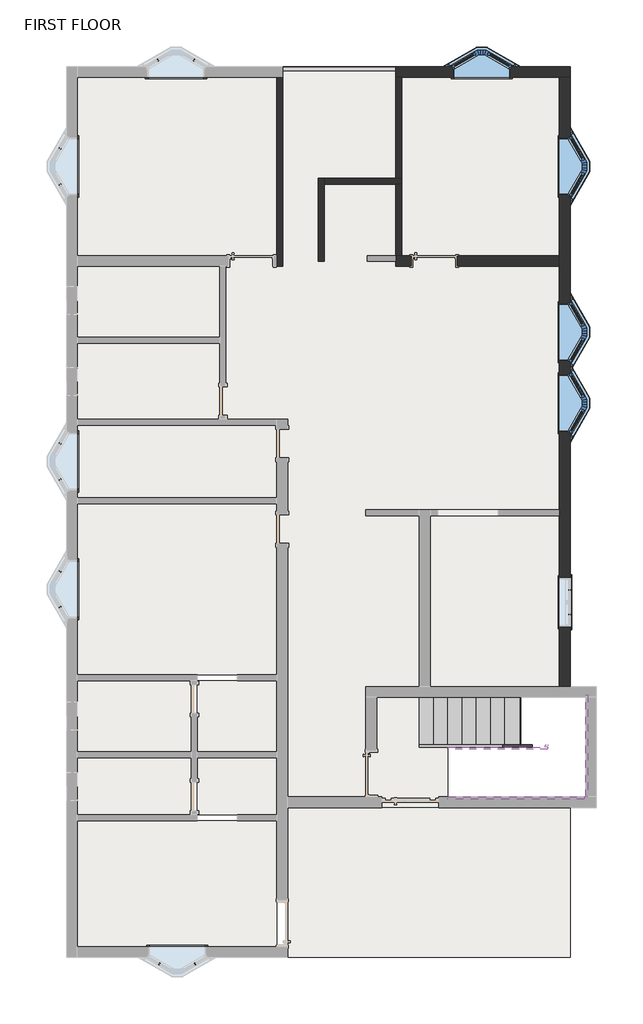
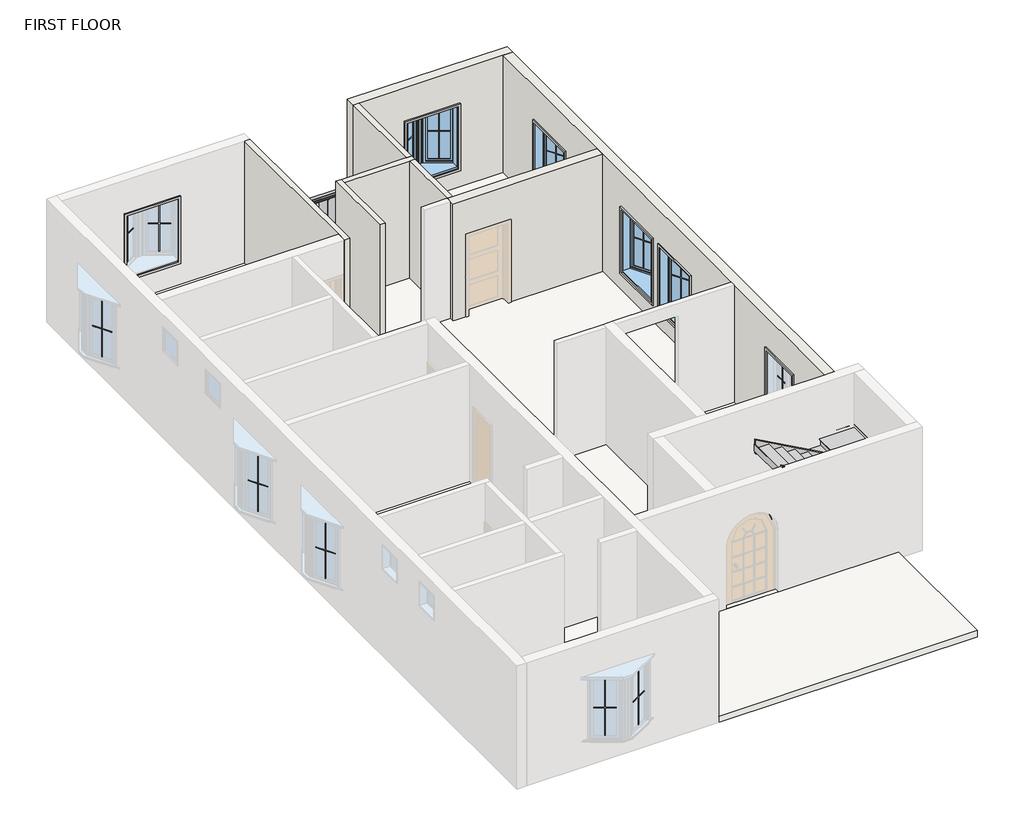
# One storey, part 2 of 2: 31 proxies, 8 walls, 6 members, 4 windows, 3 slabs, 1 railing, 1 stair flight.
"""IFC4 building model written with IfcOpenShell, lengths in millimetres."""

from ifc_helpers import new_model, si_unit, point, frame, origin, place, context, project, spatial, polyline, ellipse_curve, trimmed, outline, extrude, faceted_brep, transform, mapped, element, save
from ifc_brep_helpers import plane_surface, extruded_surface, advanced_brep
from components import muntin_pattern_2x2_muntin_pattern_2x2_75bf01dd, muntin_pattern_2x2_muntin_pattern_2x2_32baafd4, muntin_pattern_2x2_muntin_pattern_2x2_88bf7f41, muntin_pattern_2x2_muntin_pattern_2x2_3dfd0a47, trim_window_exterior_flat_with_sill_4930676f, trim_window_interior_flat_picture_frame_1060724f, trim_window_interior_flat_picture_frame_dd064338, stair_flight_7f10be43, window_bay_casement_30_degree_angle_30_angle_window_doors_2_b97d1700

model = new_model("IFC4")

# Units and contexts
model_context = context("Model", 3, world=origin())
ifc_project = project(units=[si_unit("LENGTHUNIT", "METRE", prefix="MILLI")], contexts=[model_context])

# Site, building, storey
site = spatial("IfcSite", under=ifc_project)
building = spatial("IfcBuilding", under=site)
storey = spatial("IfcBuildingStorey", under=building, Name="FIRST FLOOR", Elevation=3352.8)

# Proxies
placement = place(None, origin())
muntin_pattern_2x2_muntin_pattern_2x2_shape = muntin_pattern_2x2_muntin_pattern_2x2_75bf01dd(model_context)
element("IfcBuildingElementProxy", 1, Name="Muntin Pattern_2x2 : Muntin Pattern_2x2", ObjectType="Muntin Pattern_2x2 : Muntin Pattern_2x2", at=placement, inside=storey, context=model_context, shape_type="MappedRepresentation", body=[
    mapped(muntin_pattern_2x2_muntin_pattern_2x2_shape, transform((-20440.5197687, 51.8003691, 4083.05), x_axis=(-0.49999999999999245, 0.866025403784443, 0.0), y_axis=(-0.866025403784443, -0.49999999999999245, 0.0), z_axis=(0.0, 0.0, 1.0))),
])
element("IfcBuildingElementProxy", 2, Name="Muntin Pattern_2x2 : Muntin Pattern_2x2", ObjectType="Muntin Pattern_2x2 : Muntin Pattern_2x2", at=placement, inside=storey, context=model_context, shape_type="MappedRepresentation", body=[
    mapped(muntin_pattern_2x2_muntin_pattern_2x2_shape, transform((-20440.5197687, 2782.3003691, 4083.05), x_axis=(-0.49999999999999245, 0.866025403784443, 0.0), y_axis=(-0.866025403784443, -0.49999999999999245, 0.0), z_axis=(0.0, 0.0, 1.0))),
])
element("IfcBuildingElementProxy", 3, Name="Muntin Pattern_2x2 : Muntin Pattern_2x2", ObjectType="Muntin Pattern_2x2 : Muntin Pattern_2x2", at=placement, inside=storey, context=model_context, shape_type="MappedRepresentation", body=[
    mapped(muntin_pattern_2x2_muntin_pattern_2x2_shape, transform((-20440.5197687, 9094.2003691, 4083.05), x_axis=(-0.49999999999999245, 0.866025403784443, 0.0), y_axis=(-0.866025403784443, -0.49999999999999245, 0.0), z_axis=(0.0, 0.0, 1.0))),
])
element("IfcBuildingElementProxy", 4, Name="Muntin Pattern_2x2 : Muntin Pattern_2x2", ObjectType="Muntin Pattern_2x2 : Muntin Pattern_2x2", at=placement, inside=storey, context=model_context, shape_type="MappedRepresentation", body=[
    mapped(muntin_pattern_2x2_muntin_pattern_2x2_shape, transform((-18344.0408789, 11750.0736953, 4083.05), x_axis=(0.866025403784444, 0.49999999999999084, 0.0), y_axis=(-0.49999999999999084, 0.866025403784444, 0.0), z_axis=(0.0, 0.0, 1.0))),
])
element("IfcBuildingElementProxy", 5, Name="Muntin Pattern_2x2 : Muntin Pattern_2x2", ObjectType="Muntin Pattern_2x2 : Muntin Pattern_2x2", at=placement, inside=storey, context=model_context, shape_type="MappedRepresentation", body=[
    mapped(muntin_pattern_2x2_muntin_pattern_2x2_shape, transform((-11803.5408789, 11750.0736953, 4083.05), x_axis=(0.866025403784444, 0.49999999999999084, 0.0), y_axis=(-0.49999999999999084, 0.866025403784444, 0.0), z_axis=(0.0, 0.0, 1.0))),
])
element("IfcBuildingElementProxy", 6, Name="Muntin Pattern_2x2 : Muntin Pattern_2x2", ObjectType="Muntin Pattern_2x2 : Muntin Pattern_2x2", at=placement, inside=storey, context=model_context, shape_type="MappedRepresentation", body=[
    mapped(muntin_pattern_2x2_muntin_pattern_2x2_shape, transform((-9388.9675526, 9856.7948055, 4083.05), x_axis=(0.49999999999999245, -0.866025403784443, 0.0), y_axis=(0.866025403784443, 0.49999999999999245, 0.0), z_axis=(0.0, 0.0, 1.0))),
])
element("IfcBuildingElementProxy", 7, Name="Muntin Pattern_2x2 : Muntin Pattern_2x2", ObjectType="Muntin Pattern_2x2 : Muntin Pattern_2x2", at=placement, inside=storey, context=model_context, shape_type="MappedRepresentation", body=[
    mapped(muntin_pattern_2x2_muntin_pattern_2x2_shape, transform((-9388.9675526, 6313.4948055, 4083.05), x_axis=(0.49999999999999245, -0.866025403784443, 0.0), y_axis=(0.866025403784443, 0.49999999999999245, 0.0), z_axis=(0.0, 0.0, 1.0))),
])
element("IfcBuildingElementProxy", 8, Name="Muntin Pattern_2x2 : Muntin Pattern_2x2", ObjectType="Muntin Pattern_2x2 : Muntin Pattern_2x2", at=placement, inside=storey, context=model_context, shape_type="MappedRepresentation", body=[
    mapped(muntin_pattern_2x2_muntin_pattern_2x2_shape, transform((-9388.9675526, 4789.4948055, 4083.05), x_axis=(0.49999999999999245, -0.866025403784443, 0.0), y_axis=(0.866025403784443, 0.49999999999999245, 0.0), z_axis=(0.0, 0.0, 1.0))),
])
element("IfcBuildingElementProxy", 9, Name="Muntin Pattern_2x2 : Muntin Pattern_2x2", ObjectType="Muntin Pattern_2x2 : Muntin Pattern_2x2", at=placement, inside=storey, context=model_context, shape_type="MappedRepresentation", body=[
    mapped(muntin_pattern_2x2_muntin_pattern_2x2_shape, transform((-17556.0464424, -7581.8785207, 4083.05), x_axis=(-0.8660254037844438, -0.49999999999999106, 0.0), y_axis=(0.49999999999999106, -0.8660254037844438, 0.0), z_axis=(0.0, 0.0, 1.0))),
])
muntin_pattern_2x2_muntin_pattern_2x2_2_shape = muntin_pattern_2x2_muntin_pattern_2x2_32baafd4(model_context)
element("IfcBuildingElementProxy", 10, Name="Muntin Pattern_2x2 : Muntin Pattern_2x2", ObjectType="Muntin Pattern_2x2 : Muntin Pattern_2x2", at=placement, inside=storey, context=model_context, shape_type="MappedRepresentation", body=[
    mapped(muntin_pattern_2x2_muntin_pattern_2x2_2_shape, transform((-20440.5197687, 814.3948055, 4083.05), x_axis=(-0.4999999999999952, -0.8660254037844415, 0.0), y_axis=(0.8660254037844415, -0.4999999999999952, 0.0), z_axis=(0.0, 0.0, 1.0))),
])
element("IfcBuildingElementProxy", 11, Name="Muntin Pattern_2x2 : Muntin Pattern_2x2", ObjectType="Muntin Pattern_2x2 : Muntin Pattern_2x2", at=placement, inside=storey, context=model_context, shape_type="MappedRepresentation", body=[
    mapped(muntin_pattern_2x2_muntin_pattern_2x2_2_shape, transform((-20440.5197687, 3544.8948055, 4083.05), x_axis=(-0.4999999999999952, -0.8660254037844415, 0.0), y_axis=(0.8660254037844415, -0.4999999999999952, 0.0), z_axis=(0.0, 0.0, 1.0))),
])
element("IfcBuildingElementProxy", 12, Name="Muntin Pattern_2x2 : Muntin Pattern_2x2", ObjectType="Muntin Pattern_2x2 : Muntin Pattern_2x2", at=placement, inside=storey, context=model_context, shape_type="MappedRepresentation", body=[
    mapped(muntin_pattern_2x2_muntin_pattern_2x2_2_shape, transform((-20440.5197687, 9856.7948055, 4083.05), x_axis=(-0.4999999999999952, -0.8660254037844415, 0.0), y_axis=(0.8660254037844415, -0.4999999999999952, 0.0), z_axis=(0.0, 0.0, 1.0))),
])
element("IfcBuildingElementProxy", 13, Name="Muntin Pattern_2x2 : Muntin Pattern_2x2", ObjectType="Muntin Pattern_2x2 : Muntin Pattern_2x2", at=placement, inside=storey, context=model_context, shape_type="MappedRepresentation", body=[
    mapped(muntin_pattern_2x2_muntin_pattern_2x2_2_shape, transform((-17581.4464424, 11750.0736953, 4083.05), x_axis=(-0.8660254037844405, 0.49999999999999684, 0.0), y_axis=(-0.49999999999999684, -0.8660254037844405, 0.0), z_axis=(0.0, 0.0, 1.0))),
])
element("IfcBuildingElementProxy", 14, Name="Muntin Pattern_2x2 : Muntin Pattern_2x2", ObjectType="Muntin Pattern_2x2 : Muntin Pattern_2x2", at=placement, inside=storey, context=model_context, shape_type="MappedRepresentation", body=[
    mapped(muntin_pattern_2x2_muntin_pattern_2x2_2_shape, transform((-11040.9464424, 11750.0736953, 4083.05), x_axis=(-0.8660254037844405, 0.49999999999999684, 0.0), y_axis=(-0.49999999999999684, -0.8660254037844405, 0.0), z_axis=(0.0, 0.0, 1.0))),
])
element("IfcBuildingElementProxy", 15, Name="Muntin Pattern_2x2 : Muntin Pattern_2x2", ObjectType="Muntin Pattern_2x2 : Muntin Pattern_2x2", at=placement, inside=storey, context=model_context, shape_type="MappedRepresentation", body=[
    mapped(muntin_pattern_2x2_muntin_pattern_2x2_2_shape, transform((-9388.9675526, 9094.2003691, 4083.05), x_axis=(0.4999999999999952, 0.8660254037844415, 0.0), y_axis=(-0.8660254037844415, 0.4999999999999952, 0.0), z_axis=(0.0, 0.0, 1.0))),
])
element("IfcBuildingElementProxy", 16, Name="Muntin Pattern_2x2 : Muntin Pattern_2x2", ObjectType="Muntin Pattern_2x2 : Muntin Pattern_2x2", at=placement, inside=storey, context=model_context, shape_type="MappedRepresentation", body=[
    mapped(muntin_pattern_2x2_muntin_pattern_2x2_2_shape, transform((-9388.9675526, 5550.9003691, 4083.05), x_axis=(0.4999999999999952, 0.8660254037844415, 0.0), y_axis=(-0.8660254037844415, 0.4999999999999952, 0.0), z_axis=(0.0, 0.0, 1.0))),
])
element("IfcBuildingElementProxy", 17, Name="Muntin Pattern_2x2 : Muntin Pattern_2x2", ObjectType="Muntin Pattern_2x2 : Muntin Pattern_2x2", at=placement, inside=storey, context=model_context, shape_type="MappedRepresentation", body=[
    mapped(muntin_pattern_2x2_muntin_pattern_2x2_2_shape, transform((-9388.9675526, 4026.9003691, 4083.05), x_axis=(0.4999999999999952, 0.8660254037844415, 0.0), y_axis=(-0.8660254037844415, 0.4999999999999952, 0.0), z_axis=(0.0, 0.0, 1.0))),
])
element("IfcBuildingElementProxy", 18, Name="Muntin Pattern_2x2 : Muntin Pattern_2x2", ObjectType="Muntin Pattern_2x2 : Muntin Pattern_2x2", at=placement, inside=storey, context=model_context, shape_type="MappedRepresentation", body=[
    mapped(muntin_pattern_2x2_muntin_pattern_2x2_2_shape, transform((-18318.6408789, -7581.8785207, 4083.05), x_axis=(0.8660254037844407, -0.4999999999999966, 0.0), y_axis=(0.4999999999999966, 0.8660254037844407, 0.0), z_axis=(0.0, 0.0, 1.0))),
])
muntin_pattern_2x2_muntin_pattern_2x2_3_shape = muntin_pattern_2x2_muntin_pattern_2x2_88bf7f41(model_context)
element("IfcBuildingElementProxy", 19, Name="Muntin Pattern_2x2 : Muntin Pattern_2x2", ObjectType="Muntin Pattern_2x2 : Muntin Pattern_2x2", at=placement, inside=storey, context=model_context, shape_type="MappedRepresentation", body=[
    mapped(muntin_pattern_2x2_muntin_pattern_2x2_3_shape, transform((-9539.4686606, 412.4600873, 4337.05), x_axis=(0.0, -1.0, 0.0), y_axis=(1.0, 0.0, 0.0), z_axis=(0.0, 0.0, 1.0))),
])
muntin_pattern_2x2_muntin_pattern_2x2_4_shape = muntin_pattern_2x2_muntin_pattern_2x2_3dfd0a47(model_context)
element("IfcBuildingElementProxy", 20, Name="Muntin Pattern_2x2 : Muntin Pattern_2x2", ObjectType="Muntin Pattern_2x2 : Muntin Pattern_2x2", at=placement, inside=storey, context=model_context, shape_type="MappedRepresentation", body=[
    mapped(muntin_pattern_2x2_muntin_pattern_2x2_4_shape, transform((-9539.4686606, -105.0649127, 4337.05), x_axis=(0.0, 1.0, 0.0), y_axis=(-1.0, 0.0, 0.0), z_axis=(0.0, 0.0, 1.0))),
])
trim_window_exterior_flat_with_sill_shape = trim_window_exterior_flat_with_sill_4930676f(model_context)
element("IfcBuildingElementProxy", 21, Name="Trim-Window-Exterior-Flat : with Sill", ObjectType="Trim-Window-Exterior-Flat : with Sill", at=placement, inside=storey, context=model_context, shape_type="MappedRepresentation", body=[
    mapped(trim_window_exterior_flat_with_sill_shape, transform((-9529.9436606, 153.6975873, 5613.4), x_axis=(0.0, 1.0, 0.0), y_axis=(0.0, 0.0, 1.0), z_axis=(1.0, 0.0, 0.0))),
])
trim_window_interior_flat_picture_frame_shape = trim_window_interior_flat_picture_frame_1060724f(model_context)
element("IfcBuildingElementProxy", 22, Name="Trim-Window-Interior-Flat : Picture Frame", ObjectType="Trim-Window-Interior-Flat : Picture Frame", at=placement, inside=storey, context=model_context, shape_type="MappedRepresentation", body=[
    mapped(trim_window_interior_flat_picture_frame_shape, transform((-20070.9436606, 433.0975873, 5537.2), x_axis=(0.0, 1.0, 0.0), y_axis=(0.0, 0.0, 1.0), z_axis=(1.0, 0.0, 0.0))),
])
element("IfcBuildingElementProxy", 23, Name="Trim-Window-Interior-Flat : Picture Frame", ObjectType="Trim-Window-Interior-Flat : Picture Frame", at=placement, inside=storey, context=model_context, shape_type="MappedRepresentation", body=[
    mapped(trim_window_interior_flat_picture_frame_shape, transform((-20070.9436606, 3163.5975873, 5537.2), x_axis=(0.0, 1.0, 0.0), y_axis=(0.0, 0.0, 1.0), z_axis=(1.0, 0.0, 0.0))),
])
element("IfcBuildingElementProxy", 24, Name="Trim-Window-Interior-Flat : Picture Frame", ObjectType="Trim-Window-Interior-Flat : Picture Frame", at=placement, inside=storey, context=model_context, shape_type="MappedRepresentation", body=[
    mapped(trim_window_interior_flat_picture_frame_shape, transform((-20070.9436606, 9475.4975873, 5537.2), x_axis=(0.0, 1.0, 0.0), y_axis=(0.0, 0.0, 1.0), z_axis=(1.0, 0.0, 0.0))),
])
element("IfcBuildingElementProxy", 25, Name="Trim-Window-Interior-Flat : Picture Frame", ObjectType="Trim-Window-Interior-Flat : Picture Frame", at=placement, inside=storey, context=model_context, shape_type="MappedRepresentation", body=[
    mapped(trim_window_interior_flat_picture_frame_shape, transform((-17962.7436606, 11380.4975873, 5537.2), x_axis=(1.0, 0.0, 0.0), y_axis=(0.0, 0.0, 1.0), z_axis=(0.0, -1.0, 0.0))),
])
element("IfcBuildingElementProxy", 26, Name="Trim-Window-Interior-Flat : Picture Frame", ObjectType="Trim-Window-Interior-Flat : Picture Frame", at=placement, inside=storey, context=model_context, shape_type="MappedRepresentation", body=[
    mapped(trim_window_interior_flat_picture_frame_shape, transform((-11422.2436606, 11380.4975873, 5537.2), x_axis=(1.0, 0.0, 0.0), y_axis=(0.0, 0.0, 1.0), z_axis=(0.0, -1.0, 0.0))),
])
element("IfcBuildingElementProxy", 27, Name="Trim-Window-Interior-Flat : Picture Frame", ObjectType="Trim-Window-Interior-Flat : Picture Frame", at=placement, inside=storey, context=model_context, shape_type="MappedRepresentation", body=[
    mapped(trim_window_interior_flat_picture_frame_shape, transform((-9758.5436606, 9475.4975873, 5537.2), x_axis=(0.0, -1.0, 0.0), y_axis=(0.0, 0.0, 1.0), z_axis=(-1.0, 0.0, 0.0))),
])
element("IfcBuildingElementProxy", 28, Name="Trim-Window-Interior-Flat : Picture Frame", ObjectType="Trim-Window-Interior-Flat : Picture Frame", at=placement, inside=storey, context=model_context, shape_type="MappedRepresentation", body=[
    mapped(trim_window_interior_flat_picture_frame_shape, transform((-9758.5436606, 5932.1975873, 5537.2), x_axis=(0.0, -1.0, 0.0), y_axis=(0.0, 0.0, 1.0), z_axis=(-1.0, 0.0, 0.0))),
])
element("IfcBuildingElementProxy", 29, Name="Trim-Window-Interior-Flat : Picture Frame", ObjectType="Trim-Window-Interior-Flat : Picture Frame", at=placement, inside=storey, context=model_context, shape_type="MappedRepresentation", body=[
    mapped(trim_window_interior_flat_picture_frame_shape, transform((-9758.5436606, 4408.1975873, 5537.2), x_axis=(0.0, -1.0, 0.0), y_axis=(0.0, 0.0, 1.0), z_axis=(-1.0, 0.0, 0.0))),
])
element("IfcBuildingElementProxy", 30, Name="Trim-Window-Interior-Flat : Picture Frame", ObjectType="Trim-Window-Interior-Flat : Picture Frame", at=placement, inside=storey, context=model_context, shape_type="MappedRepresentation", body=[
    mapped(trim_window_interior_flat_picture_frame_shape, transform((-17937.3436606, -7212.3024127, 5537.2), x_axis=(-1.0, 0.0, 0.0), y_axis=(0.0, 0.0, 1.0), z_axis=(0.0, 1.0, 0.0))),
])
trim_window_interior_flat_picture_frame_2_shape = trim_window_interior_flat_picture_frame_dd064338(model_context)
element("IfcBuildingElementProxy", 31, Name="Trim-Window-Interior-Flat : Picture Frame", ObjectType="Trim-Window-Interior-Flat : Picture Frame", at=placement, inside=storey, context=model_context, shape_type="MappedRepresentation", body=[
    mapped(trim_window_interior_flat_picture_frame_2_shape, transform((-9758.5436606, 153.6975873, 5613.4), x_axis=(0.0, -1.0, 0.0), y_axis=(0.0, 0.0, 1.0), z_axis=(-1.0, 0.0, 0.0))),
])

# Members
element("IfcMember", 32, ObjectType="Stringer - 2\" Width", at=placement, inside=storey, context=model_context, shape_type="SweptSolid", body=[
    extrude(outline(polyline([(3560.3983948, -12755.7436606), (3352.8, -12755.7436606), (3352.8, -12501.7991578), (5122.3333333, -9316.6391578), (5122.3333333, -9944.2607712), (3560.3983948, -12755.7436606)])), frame((0.0, -1878.3024127, 0.0), z_axis=(0.0, 1.0, 0.0), x_axis=(0.0, 0.0, 1.0)), (0.0, 0.0, 1.0), 50.8),
])
element("IfcMember", 33, ObjectType="Stringer - 2\" Width", at=placement, inside=storey, context=model_context, shape_type="SweptSolid", body=[
    extrude(outline(polyline([(-9199.7436606, -1827.5024127), (-9148.9436606, -1827.5024127), (-9148.9436606, -4011.9024127), (-9199.7436606, -4011.9024127), (-9199.7436606, -1827.5024127)])), frame((0.0, 0.0, 4817.5333333), z_axis=(0.0, 0.0, 1.0), x_axis=(1.0, 0.0, 0.0)), (0.0, 0.0, 1.0), 304.8),
])
element("IfcMember", 34, ObjectType="Stringer - 2\" Width", at=placement, inside=storey, context=model_context, shape_type="SweptSolid", body=[
    extrude(outline(polyline([(4817.5333333, -9227.38655), (6439.0650614, -12146.1436606), (6090.3863873, -12146.1436606), (4817.5333333, -9855.0081634), (4817.5333333, -9227.38655)])), frame((0.0, -4062.7024127, 0.0), z_axis=(0.0, 1.0, 0.0), x_axis=(0.0, 0.0, 1.0)), (0.0, 0.0, 1.0), 50.8),
])
element("IfcMember", 35, ObjectType="Stringer - 2\" Width", at=placement, inside=storey, context=model_context, shape_type="SweptSolid", body=[
    extrude(outline(polyline([(3560.3983948, -12755.7436606), (3352.8, -12755.7436606), (3352.8, -12501.7991578), (4707.4974985, -10063.3436606), (5056.1761726, -10063.3436606), (3560.3983948, -12755.7436606)])), frame((0.0, -2945.1024127, 0.0), z_axis=(0.0, 1.0, 0.0), x_axis=(0.0, 0.0, 1.0)), (0.0, 0.0, 1.0), 50.8),
])
element("IfcMember", 36, ObjectType="Stringer - 2\" Width", at=placement, inside=storey, context=model_context, shape_type="SweptSolid", body=[
    extrude(outline(polyline([(-10063.3436606, -2894.3024127), (-10012.5436606, -2894.3024127), (-10012.5436606, -2945.1024127), (-10063.3436606, -2945.1024127), (-10063.3436606, -2894.3024127)])), frame((0.0, 0.0, 4817.5333333), z_axis=(0.0, 0.0, 1.0), x_axis=(1.0, 0.0, 0.0)), (0.0, 0.0, 1.0), 304.8),
])
element("IfcMember", 37, ObjectType="Stringer - 2\" Width", at=placement, inside=storey, context=model_context, shape_type="SweptSolid", body=[
    extrude(outline(polyline([(4905.053054, -10012.5436606), (5253.7317281, -10012.5436606), (6439.0650614, -12146.1436606), (6090.3863873, -12146.1436606), (4905.053054, -10012.5436606)])), frame((0.0, -2995.9024127, 0.0), z_axis=(0.0, 1.0, 0.0), x_axis=(0.0, 0.0, 1.0)), (0.0, 0.0, 1.0), 50.8),
])

# Railing
element("IfcRailing", 38, ObjectType="Glass Panel - Bottom Fill", at=placement, inside=storey, context=model_context, shape_type="SolidModel", body=[
    advanced_brep(
    [(-13263.7436606, 11520.1975873, 4267.2), (-13263.7436606, 11596.3975873, 4267.2), (-15676.7436606, 11520.1975873, 4267.2), (-15676.7436606, 11596.3975873, 4267.2)],
    [
        (0, 1, ellipse_curve(frame((-13263.7436606, 11558.2975873, 4267.2), z_axis=(1.0, 0.0, 0.0), x_axis=(0.0, 1.0, 0.0)), 38.1, 28.575)),
        (1, 0, ellipse_curve(frame((-13263.7436606, 11558.2975873, 4267.2), z_axis=(1.0, 0.0, 0.0), x_axis=(0.0, 1.0, 0.0)), 38.1, 28.575)),
        (2, 3, ellipse_curve(frame((-15676.7436606, 11558.2975873, 4267.2), z_axis=(-1.0, 0.0, 0.0), x_axis=(0.0, 1.0, 0.0)), 38.1, 28.575)),
        (3, 2, ellipse_curve(frame((-15676.7436606, 11558.2975873, 4267.2), z_axis=(-1.0, 0.0, 0.0), x_axis=(0.0, 1.0, 0.0)), 38.1, 28.575)),
        (0, 2),
        (3, 1),
    ],
    [
        plane_surface(frame((-13263.7436606, 11558.2975873, 4267.2), z_axis=(1.0, 0.0, 0.0), x_axis=(0.0, -1.0, 0.0))),
        plane_surface(frame((-15676.7436606, 11558.2975873, 4267.2), z_axis=(-1.0, 0.0, 0.0), x_axis=(0.0, -1.0, 0.0))),
        extruded_surface(trimmed(ellipse_curve(frame((-15676.7436606, 11558.2975873, 4267.2), z_axis=(1.0, 0.0, 0.0), x_axis=(0.0, 1.0, 0.0)), 38.1, 28.575), [point((-15676.7436606, 11520.1975873, 4267.2))], [point((-15676.7436606, 11596.3975873, 4267.2))], True, "CARTESIAN"), (2413.0, 0.0, 0.0), 2413.0),
        extruded_surface(trimmed(ellipse_curve(frame((-15676.7436606, 11558.2975873, 4267.2), z_axis=(1.0, 0.0, 0.0), x_axis=(0.0, 1.0, 0.0)), 38.1, 28.575), [point((-15676.7436606, 11596.3975873, 4267.2))], [point((-15676.7436606, 11520.1975873, 4267.2))], True, "CARTESIAN"), (2413.0, 0.0, 0.0), 2413.0),
    ],
    [
        (0, [[1, 2]]),
        (1, [[3, 4]]),
        (2, [[-1, 5, -4, 6]]),
        (3, [[-2, -6, -3, -5]]),
    ],
),
    extrude(outline(polyline([(-13263.7436606, 11570.9975873), (-13263.7436606, 11545.5975873), (-15676.7436606, 11545.5975873), (-15676.7436606, 11570.9975873), (-13263.7436606, 11570.9975873)])), frame((0.0, 0.0, 4152.9), z_axis=(0.0, 0.0, 1.0), x_axis=(1.0, 0.0, 0.0)), (0.0, 0.0, 1.0), 25.4),
    extrude(outline(polyline([(-15181.4436606, 11551.9475873), (-15791.0436606, 11551.9475873), (-15791.0436606, 11558.2975873), (-15181.4436606, 11558.2975873), (-15181.4436606, 11551.9475873)])), frame((0.0, 0.0, 3479.8), z_axis=(0.0, 0.0, 1.0), x_axis=(1.0, 0.0, 0.0)), (0.0, 0.0, 1.0), 647.7),
    extrude(outline(polyline([(-14775.0436606, 11551.9475873), (-15384.6436606, 11551.9475873), (-15384.6436606, 11558.2975873), (-14775.0436606, 11558.2975873), (-14775.0436606, 11551.9475873)])), frame((0.0, 0.0, 3479.8), z_axis=(0.0, 0.0, 1.0), x_axis=(1.0, 0.0, 0.0)), (0.0, 0.0, 1.0), 647.7),
    extrude(outline(polyline([(-14368.6436606, 11551.9475873), (-14978.2436606, 11551.9475873), (-14978.2436606, 11558.2975873), (-14368.6436606, 11558.2975873), (-14368.6436606, 11551.9475873)])), frame((0.0, 0.0, 3479.8), z_axis=(0.0, 0.0, 1.0), x_axis=(1.0, 0.0, 0.0)), (0.0, 0.0, 1.0), 647.7),
    extrude(outline(polyline([(-13962.2436606, 11551.9475873), (-14571.8436606, 11551.9475873), (-14571.8436606, 11558.2975873), (-13962.2436606, 11558.2975873), (-13962.2436606, 11551.9475873)])), frame((0.0, 0.0, 3479.8), z_axis=(0.0, 0.0, 1.0), x_axis=(1.0, 0.0, 0.0)), (0.0, 0.0, 1.0), 647.7),
    extrude(outline(polyline([(-13555.8436606, 11551.9475873), (-14165.4436606, 11551.9475873), (-14165.4436606, 11558.2975873), (-13555.8436606, 11558.2975873), (-13555.8436606, 11551.9475873)])), frame((0.0, 0.0, 3479.8), z_axis=(0.0, 0.0, 1.0), x_axis=(1.0, 0.0, 0.0)), (0.0, 0.0, 1.0), 647.7),
    extrude(outline(polyline([(-13149.4436606, 11551.9475873), (-13759.0436606, 11551.9475873), (-13759.0436606, 11558.2975873), (-13149.4436606, 11558.2975873), (-13149.4436606, 11551.9475873)])), frame((0.0, 0.0, 3479.8), z_axis=(0.0, 0.0, 1.0), x_axis=(1.0, 0.0, 0.0)), (0.0, 0.0, 1.0), 647.7),
])

# Slabs
element("IfcSlab", 39, at=placement, inside=storey, context=model_context, shape_type="SweptSolid", body=[
    extrude(outline(polyline([(-15803.7436606, 11380.4975873), (-15803.7436606, 7570.4975873), (-20070.9436606, 7570.4975873), (-20070.9436606, 11380.4975873), (-15803.7436606, 11380.4975873)])), frame((0.0, 0.0, 3225.8), z_axis=(0.0, 0.0, 1.0), x_axis=(1.0, 0.0, 0.0)), (0.0, 0.0, 1.0), 152.4),
])
element("IfcSlab", 40, at=placement, inside=storey, context=model_context, shape_type="SweptSolid", body=[
    extrude(outline(polyline([(-17022.9436606, 7341.8975873), (-17022.9436606, 5817.8975873), (-20070.9436606, 5817.8975873), (-20070.9436606, 7341.8975873), (-17022.9436606, 7341.8975873)])), frame((0.0, 0.0, 3352.8), z_axis=(0.0, 0.0, 1.0), x_axis=(1.0, 0.0, 0.0)), (0.0, 0.0, 1.0), 152.4),
    extrude(outline(polyline([(-17022.9436606, 5690.8975873), (-17022.9436606, 4065.2975873), (-20070.9436606, 4065.2975873), (-20070.9436606, 5690.8975873), (-17022.9436606, 5690.8975873)])), frame((0.0, 0.0, 3352.8), z_axis=(0.0, 0.0, 1.0), x_axis=(1.0, 0.0, 0.0)), (0.0, 0.0, 1.0), 152.4),
    extrude(outline(polyline([(-15803.7436606, 3938.2975873), (-15803.7436606, 2388.8975873), (-20070.9436606, 2388.8975873), (-20070.9436606, 3938.2975873), (-15803.7436606, 3938.2975873)])), frame((0.0, 0.0, 3352.8), z_axis=(0.0, 0.0, 1.0), x_axis=(1.0, 0.0, 0.0)), (0.0, 0.0, 1.0), 152.4),
    extrude(outline(polyline([(-15803.7436606, 2261.8975873), (-15803.7436606, -1395.7024127), (-20070.9436606, -1395.7024127), (-20070.9436606, 2261.8975873), (-15803.7436606, 2261.8975873)])), frame((0.0, 0.0, 3352.8), z_axis=(0.0, 0.0, 1.0), x_axis=(1.0, 0.0, 0.0)), (0.0, 0.0, 1.0), 152.4),
    extrude(outline(polyline([(-17632.5436606, -1522.7024127), (-17632.5436606, -3046.7024127), (-20070.9436606, -3046.7024127), (-20070.9436606, -1522.7024127), (-17632.5436606, -1522.7024127)])), frame((0.0, 0.0, 3352.8), z_axis=(0.0, 0.0, 1.0), x_axis=(1.0, 0.0, 0.0)), (0.0, 0.0, 1.0), 152.4),
    extrude(outline(polyline([(-17505.5436606, -3046.7024127), (-17505.5436606, -1522.7024127), (-15803.7436606, -1522.7024127), (-15803.7436606, -3046.7024127), (-17505.5436606, -3046.7024127)])), frame((0.0, 0.0, 3352.8), z_axis=(0.0, 0.0, 1.0), x_axis=(1.0, 0.0, 0.0)), (0.0, 0.0, 1.0), 152.4),
    extrude(outline(polyline([(-17632.5436606, -3173.7024127), (-17632.5436606, -4392.9024127), (-20070.9436606, -4392.9024127), (-20070.9436606, -3173.7024127), (-17632.5436606, -3173.7024127)])), frame((0.0, 0.0, 3352.8), z_axis=(0.0, 0.0, 1.0), x_axis=(1.0, 0.0, 0.0)), (0.0, 0.0, 1.0), 152.4),
    extrude(outline(polyline([(-15803.7436606, -3173.7024127), (-15803.7436606, -4392.9024127), (-17505.5436606, -4392.9024127), (-17505.5436606, -3173.7024127), (-15803.7436606, -3173.7024127)])), frame((0.0, 0.0, 3352.8), z_axis=(0.0, 0.0, 1.0), x_axis=(1.0, 0.0, 0.0)), (0.0, 0.0, 1.0), 152.4),
    extrude(outline(polyline([(-15803.7436606, -4519.9024127), (-15803.7436606, -7212.3024127), (-20070.9436606, -7212.3024127), (-20070.9436606, -4519.9024127), (-15803.7436606, -4519.9024127)])), frame((0.0, 0.0, 3352.8), z_axis=(0.0, 0.0, 1.0), x_axis=(1.0, 0.0, 0.0)), (0.0, 0.0, 1.0), 152.4),
    extrude(outline(polyline([(-9758.5436606, 2007.8975873), (-9758.5436606, -1649.7024127), (-12527.1436606, -1649.7024127), (-12527.1436606, 2007.8975873), (-9758.5436606, 2007.8975873)])), frame((0.0, 0.0, 3352.8), z_axis=(0.0, 0.0, 1.0), x_axis=(1.0, 0.0, 0.0)), (0.0, 0.0, 1.0), 152.4),
    extrude(outline(polyline([(-9758.5436606, 11380.4975873), (-9758.5436606, 7570.4975873), (-13136.7436606, 7570.4975873), (-13136.7436606, 11380.4975873), (-9758.5436606, 11380.4975873)])), frame((0.0, 0.0, 3352.8), z_axis=(0.0, 0.0, 1.0), x_axis=(1.0, 0.0, 0.0)), (0.0, 0.0, 1.0), 152.4),
    extrude(outline(polyline([(-9529.9436606, -4240.5024127), (-9529.9436606, -7440.9024127), (-15575.1436606, -7440.9024127), (-15575.1436606, -4240.5024127), (-9529.9436606, -4240.5024127)])), frame((0.0, 0.0, 3352.8), z_axis=(0.0, 0.0, 1.0), x_axis=(1.0, 0.0, 0.0)), (0.0, 0.0, 1.0), 152.4),
])
element("IfcSlab", 41, at=placement, inside=storey, context=model_context, shape_type="SweptSolid", body=[
    extrude(outline(polyline([(-13263.7436606, 11609.0975873), (-13263.7436606, 9221.4975873), (-14914.7436606, 9221.4975873), (-14914.7436606, 7443.4975873), (-14787.7436606, 7443.4975873), (-14787.7436606, 9094.4975873), (-13263.7436606, 9094.4975873), (-13263.7436606, 7570.4975873), (-13873.3436606, 7570.4975873), (-13873.3436606, 7443.4975873), (-13263.7436606, 7443.4975873), (-13263.7436606, 7341.8975873), (-12920.8436606, 7341.8975873), (-12920.8436606, 7570.4975873), (-11955.6436606, 7570.4975873), (-11955.6436606, 7341.8975873), (-9758.5436606, 7341.8975873), (-9758.5436606, 2134.8975873), (-13898.7436606, 2134.8975873), (-13898.7436606, 2007.8975873), (-12755.7436606, 2007.8975873), (-12755.7436606, -1649.7024127), (-13898.7436606, -1649.7024127), (-13898.7436606, -3034.0024127), (-13670.1436606, -3034.0024127), (-13670.1436606, -1878.3024127), (-12755.7436606, -1878.3024127), (-12755.7436606, -2945.1024127), (-12146.1436606, -2945.1024127), (-12146.1436606, -4011.9024127), (-12336.6436606, -4011.9024127), (-12336.6436606, -4240.5024127), (-13555.8436606, -4240.5024127), (-13555.8436606, -4011.9024127), (-15575.1436606, -4011.9024127), (-15575.1436606, 1410.9975873), (-15803.7436606, 1410.9975873), (-15803.7436606, 2022.2890433), (-15575.1436606, 2022.2890433), (-15575.1436606, 3239.7975873), (-15803.7436606, 3239.7975873), (-15803.7436606, 3849.3975873), (-15575.1436606, 3849.3975873), (-15575.1436606, 4065.2975873), (-16895.9436606, 4065.2975873), (-16895.9436606, 4154.1975873), (-17022.9436606, 4154.1975873), (-17022.9436606, 4763.7975873), (-16895.9436606, 4763.7975873), (-16895.9436606, 7341.8975873), (-16832.4436606, 7341.8975873), (-16832.4436606, 7570.4975873), (-15867.2436606, 7570.4975873), (-15867.2436606, 7341.8975873), (-15676.7436606, 7341.8975873), (-15676.7436606, 11609.0975873), (-13263.7436606, 11609.0975873)])), frame((0.0, 0.0, 3352.8), z_axis=(0.0, 0.0, 1.0), x_axis=(1.0, 0.0, 0.0)), (0.0, 0.0, 1.0), 152.4),
])

# Stair flight
stair_flight_shape = stair_flight_7f10be43(model_context)
element("IfcStairFlight", 42, ObjectType="2\" Tread 1\" Nosing 1/4\" Riser", at=placement, inside=storey, context=model_context, shape_type="MappedRepresentation", body=[
    mapped(stair_flight_shape, transform((0.0, 0.0, 0.0), x_axis=(1.0, 0.0, 0.0), y_axis=(0.0, 1.0, 0.0), z_axis=(0.0, 0.0, 1.0))),
])

# Walls
element("IfcWall", 43, at=placement, inside=storey, context=model_context, shape_type="Brep", body=[
    faceted_brep([(-13263.7436606, 11380.4975873, 3352.8), (-13136.7436606, 11380.4975873, 3352.8), (-9758.5436606, 11380.4975873, 3352.8), (-9529.9436606, 11380.4975873, 3352.8), (-9529.9436606, 11380.4975873, 6400.8), (-9758.5436606, 11380.4975873, 6400.8), (-13136.7436606, 11380.4975873, 6400.8), (-13263.7436606, 11380.4975873, 6400.8), (-12031.8436606, 11380.4975873, 5537.2), (-10812.6436606, 11380.4975873, 5537.2), (-10812.6436606, 11380.4975873, 3962.4), (-12031.8436606, 11380.4975873, 3962.4), (-13263.7436606, 11609.0975873, 3352.8), (-13263.7436606, 11609.0975873, 6400.8), (-9529.9436606, 11609.0975873, 6400.8), (-9529.9436606, 11609.0975873, 3352.8), (-10777.7186606, 11609.0975873, 5537.2), (-12066.7686606, 11609.0975873, 5537.2), (-12066.7686606, 11609.0975873, 3962.4), (-10777.7186606, 11609.0975873, 3962.4), (-12031.8436606, 11548.6057128, 5537.2), (-10812.6436606, 11548.6057128, 5537.2), (-12031.8436606, 11548.6057128, 3962.4), (-10812.6436606, 11548.6057128, 3962.4)], [[[0, 1, 2, 3, 4, 5, 6, 7], [8, 9, 10, 11]], [[12, 13, 14, 15], [16, 17, 18, 19]], [[3, 2, 1, 0, 12, 15]], [[7, 6, 5, 4, 14, 13]], [[4, 3, 15, 14]], [[0, 7, 13, 12]], [[20, 17, 16, 21, 9, 8]], [[22, 11, 10, 23, 19, 18]], [[20, 8, 11, 22]], [[9, 21, 23, 10]], [[21, 16, 19, 23]], [[17, 20, 22, 18]]]),
])
element("IfcWall", 44, at=placement, inside=storey, context=model_context, shape_type="Brep", body=[
    faceted_brep([(-9758.5436606, 11380.4975873, 3352.8), (-9758.5436606, 7570.4975873, 3352.8), (-9758.5436606, 7341.8975873, 3352.8), (-9758.5436606, 2134.8975873, 3352.8), (-9758.5436606, 2007.8975873, 3352.8), (-9758.5436606, -1649.7024127, 3352.8), (-9758.5436606, -1649.7024127, 6400.8), (-9758.5436606, 2007.8975873, 6400.8), (-9758.5436606, 2134.8975873, 6400.8), (-9758.5436606, 7341.8975873, 6400.8), (-9758.5436606, 7570.4975873, 6400.8), (-9758.5436606, 11380.4975873, 6400.8), (-9758.5436606, 10085.0975873, 5537.2), (-9758.5436606, 8865.8975873, 5537.2), (-9758.5436606, 8865.8975873, 3962.4), (-9758.5436606, 10085.0975873, 3962.4), (-9758.5436606, 6541.7975873, 5537.2), (-9758.5436606, 5322.5975873, 5537.2), (-9758.5436606, 5322.5975873, 3962.4), (-9758.5436606, 6541.7975873, 3962.4), (-9758.5436606, 5017.7975873, 5537.2), (-9758.5436606, 3798.5975873, 5537.2), (-9758.5436606, 3798.5975873, 3962.4), (-9758.5436606, 5017.7975873, 3962.4), (-9758.5436606, -367.0024127, 5613.4), (-9758.5436606, -367.0024127, 4267.2), (-9758.5436606, 674.3975873, 4267.2), (-9758.5436606, 674.3975873, 5613.4), (-9529.9436606, 11380.4975873, 3352.8), (-9529.9436606, 11380.4975873, 6400.8), (-9529.9436606, -1649.7024127, 6400.8), (-9529.9436606, -1649.7024127, 3352.8), (-9529.9436606, 8830.9725873, 5537.2), (-9529.9436606, 10120.0225873, 5537.2), (-9529.9436606, 10120.0225873, 3962.4), (-9529.9436606, 8830.9725873, 3962.4), (-9529.9436606, 5287.6725873, 5537.2), (-9529.9436606, 6576.7225873, 5537.2), (-9529.9436606, 6576.7225873, 3962.4), (-9529.9436606, 5287.6725873, 3962.4), (-9529.9436606, 3763.6725873, 5537.2), (-9529.9436606, 5052.7225873, 5537.2), (-9529.9436606, 5052.7225873, 3962.4), (-9529.9436606, 3763.6725873, 3962.4), (-9529.9436606, -367.0024127, 5613.4), (-9529.9436606, 674.3975873, 5613.4), (-9529.9436606, 674.3975873, 4267.2), (-9529.9436606, -367.0024127, 4267.2), (-9590.4355351, 10085.0975873, 5537.2), (-9590.4355351, 8865.8975873, 5537.2), (-9590.4355351, 10085.0975873, 3962.4), (-9590.4355351, 8865.8975873, 3962.4), (-9590.4355351, 6541.7975873, 5537.2), (-9590.4355351, 5322.5975873, 5537.2), (-9590.4355351, 6541.7975873, 3962.4), (-9590.4355351, 5322.5975873, 3962.4), (-9590.4355351, 5017.7975873, 5537.2), (-9590.4355351, 3798.5975873, 5537.2), (-9590.4355351, 5017.7975873, 3962.4), (-9590.4355351, 3798.5975873, 3962.4)], [[[0, 1, 2, 3, 4, 5, 6, 7, 8, 9, 10, 11], [12, 13, 14, 15], [16, 17, 18, 19], [20, 21, 22, 23], [24, 25, 26, 27]], [[28, 29, 30, 31], [32, 33, 34, 35], [36, 37, 38, 39], [40, 41, 42, 43], [44, 45, 46, 47]], [[5, 4, 3, 2, 1, 0, 28, 31]], [[11, 10, 9, 8, 7, 6, 30, 29]], [[0, 11, 29, 28]], [[6, 5, 31, 30]], [[48, 33, 32, 49, 13, 12]], [[50, 15, 14, 51, 35, 34]], [[48, 12, 15, 50]], [[13, 49, 51, 14]], [[49, 32, 35, 51]], [[33, 48, 50, 34]], [[52, 37, 36, 53, 17, 16]], [[54, 19, 18, 55, 39, 38]], [[52, 16, 19, 54]], [[17, 53, 55, 18]], [[53, 36, 39, 55]], [[37, 52, 54, 38]], [[56, 41, 40, 57, 21, 20]], [[58, 23, 22, 59, 43, 42]], [[56, 20, 23, 58]], [[21, 57, 59, 22]], [[57, 40, 43, 59]], [[41, 56, 58, 42]], [[25, 24, 44, 47]], [[26, 25, 47, 46]], [[27, 26, 46, 45]], [[24, 27, 45, 44]]]),
])
element("IfcWall", 45, at=placement, inside=storey, context=model_context, shape_type="Brep", body=[
    faceted_brep([(-13263.7436606, 7570.4975873, 6400.8), (-13136.7436606, 7570.4975873, 6400.8), (-9758.5436606, 7570.4975873, 6400.8), (-9758.5436606, 7570.4975873, 3352.8), (-11955.6436606, 7570.4975873, 3352.8), (-11955.6436606, 7570.4975873, 5511.8), (-12920.8436606, 7570.4975873, 5511.8), (-12920.8436606, 7570.4975873, 3352.8), (-13136.7436606, 7570.4975873, 3352.8), (-13263.7436606, 7570.4975873, 3352.8), (-9758.5436606, 7341.8975873, 6400.8), (-13263.7436606, 7341.8975873, 6400.8), (-13263.7436606, 7341.8975873, 3352.8), (-12920.8436606, 7341.8975873, 3352.8), (-12920.8436606, 7341.8975873, 5511.8), (-11955.6436606, 7341.8975873, 5511.8), (-11955.6436606, 7341.8975873, 3352.8), (-9758.5436606, 7341.8975873, 3352.8), (-13263.7436606, 7443.4975873, 3352.8), (-13263.7436606, 7443.4975873, 6400.8)], [[[0, 1, 2, 3, 4, 5, 6, 7, 8, 9]], [[10, 11, 12, 13, 14, 15, 16, 17]], [[3, 17, 16, 4]], [[12, 18, 9, 8, 7, 13]], [[2, 1, 0, 19, 11, 10]], [[3, 2, 10, 17]], [[0, 9, 18, 12, 11, 19]], [[15, 5, 4, 16]], [[5, 15, 14, 6]], [[6, 14, 13, 7]]]),
])
element("IfcWall", 46, ObjectType="INNER WALL 5\"", at=placement, inside=storey, context=model_context, shape_type="Brep", body=[
    faceted_brep([(-15803.7436606, 11380.4975873, 3352.8), (-15803.7436606, 7570.4975873, 3352.8), (-15803.7436606, 7341.8975873, 3352.8), (-15803.7436606, 7341.8975873, 6400.8), (-15803.7436606, 7570.4975873, 6400.8), (-15803.7436606, 11380.4975873, 6400.8), (-15676.7436606, 11380.4975873, 3352.8), (-15676.7436606, 11380.4975873, 6400.8), (-15676.7436606, 7341.8975873, 6400.8), (-15676.7436606, 7341.8975873, 3352.8)], [[[0, 1, 2, 3, 4, 5]], [[6, 7, 8, 9]], [[2, 1, 0, 6, 9]], [[5, 4, 3, 8, 7]], [[0, 5, 7, 6]], [[3, 2, 9, 8]]]),
])
element("IfcWall", 47, ObjectType="INNER WALL 5\"", at=placement, inside=storey, context=model_context, shape_type="Brep", body=[
    faceted_brep([(-14787.7436606, 7443.4975873, 3352.8), (-14787.7436606, 9094.4975873, 3352.8), (-14787.7436606, 9221.4975873, 3352.8), (-14787.7436606, 9221.4975873, 6400.8), (-14787.7436606, 9094.4975873, 6400.8), (-14787.7436606, 7443.4975873, 6400.8), (-14914.7436606, 7443.4975873, 3352.8), (-14914.7436606, 7443.4975873, 6400.8), (-14914.7436606, 9221.4975873, 6400.8), (-14914.7436606, 9221.4975873, 3352.8)], [[[0, 1, 2, 3, 4, 5]], [[6, 7, 8, 9]], [[2, 1, 0, 6, 9]], [[5, 4, 3, 8, 7]], [[0, 5, 7, 6]], [[3, 2, 9, 8]]]),
])
element("IfcWall", 48, ObjectType="INNER WALL 5\"", at=placement, inside=storey, context=model_context, shape_type="Brep", body=[
    faceted_brep([(-14787.7436606, 9094.4975873, 3352.8), (-13263.7436606, 9094.4975873, 3352.8), (-13136.7436606, 9094.4975873, 3352.8), (-13136.7436606, 9094.4975873, 6400.8), (-13263.7436606, 9094.4975873, 6400.8), (-14787.7436606, 9094.4975873, 6400.8), (-14787.7436606, 9221.4975873, 3352.8), (-14787.7436606, 9221.4975873, 6400.8), (-13263.7436606, 9221.4975873, 6400.8), (-13136.7436606, 9221.4975873, 6400.8), (-13136.7436606, 9221.4975873, 3352.8), (-13263.7436606, 9221.4975873, 3352.8)], [[[0, 1, 2, 3, 4, 5]], [[6, 7, 8, 9, 10, 11]], [[2, 1, 0, 6, 11, 10]], [[5, 4, 3, 9, 8, 7]], [[0, 5, 7, 6]], [[3, 2, 10, 9]]]),
])
element("IfcWall", 49, ObjectType="INNER WALL 5\"", at=placement, inside=storey, context=model_context, shape_type="SweptSolid", body=[
    extrude(outline(polyline([(-13136.7436606, 11380.4975873), (-13136.7436606, 9221.4975873), (-13263.7436606, 9221.4975873), (-13263.7436606, 11380.4975873), (-13136.7436606, 11380.4975873)])), frame((0.0, 0.0, 3352.8), z_axis=(0.0, 0.0, 1.0), x_axis=(1.0, 0.0, 0.0)), (0.0, 0.0, 1.0), 3048.0),
])
element("IfcWall", 50, ObjectType="INNER WALL 5\"", at=placement, inside=storey, context=model_context, shape_type="SweptSolid", body=[
    extrude(outline(polyline([(-13263.7436606, 7570.4975873), (-13263.7436606, 9094.4975873), (-13136.7436606, 9094.4975873), (-13136.7436606, 7570.4975873), (-13263.7436606, 7570.4975873)])), frame((0.0, 0.0, 3352.8), z_axis=(0.0, 0.0, 1.0), x_axis=(1.0, 0.0, 0.0)), (0.0, 0.0, 1.0), 3048.0),
])

# Windows
window_bay_casement_30_degree_angle_30_angle_window_doors_2_shape = window_bay_casement_30_degree_angle_30_angle_window_doors_2_b97d1700(model_context)
element("IfcWindow", 51, ObjectType="Window-Bay-Casement-30_Degree_Angle : 30 ANGLE WINDOW DOORS", at=placement, inside=storey, context=model_context, shape_type="MappedRepresentation", body=[
    mapped(window_bay_casement_30_degree_angle_30_angle_window_doors_2_shape, transform((-11422.2436606, 11494.7975873, 3352.8), x_axis=(1.0, 0.0, 0.0), y_axis=(0.0, 1.0, 0.0), z_axis=(0.0, 0.0, 1.0))),
])
element("IfcWindow", 52, ObjectType="Window-Bay-Casement-30_Degree_Angle : 30 ANGLE WINDOW DOORS", at=placement, inside=storey, context=model_context, shape_type="MappedRepresentation", body=[
    mapped(window_bay_casement_30_degree_angle_30_angle_window_doors_2_shape, transform((-9644.2436606, 9475.4975873, 3352.8), x_axis=(0.0, -1.0, 0.0), y_axis=(1.0, 0.0, 0.0), z_axis=(0.0, 0.0, 1.0))),
])
element("IfcWindow", 53, ObjectType="Window-Bay-Casement-30_Degree_Angle : 30 ANGLE WINDOW DOORS", at=placement, inside=storey, context=model_context, shape_type="MappedRepresentation", body=[
    mapped(window_bay_casement_30_degree_angle_30_angle_window_doors_2_shape, transform((-9644.2436606, 5932.1975873, 3352.8), x_axis=(0.0, -1.0, 0.0), y_axis=(1.0, 0.0, 0.0), z_axis=(0.0, 0.0, 1.0))),
])
element("IfcWindow", 54, ObjectType="Window-Bay-Casement-30_Degree_Angle : 30 ANGLE WINDOW DOORS", at=placement, inside=storey, context=model_context, shape_type="MappedRepresentation", body=[
    mapped(window_bay_casement_30_degree_angle_30_angle_window_doors_2_shape, transform((-9644.2436606, 4408.1975873, 3352.8), x_axis=(0.0, -1.0, 0.0), y_axis=(1.0, 0.0, 0.0), z_axis=(0.0, 0.0, 1.0))),
])

save(model, "model.ifc")

# Revit data of these elements
# Type "Muntin Pattern_2x2 : Muntin Pattern_2x2"
#   Width [instance default] = 4' - 0"
#   Thickness = 0' - 0 1/2"
#   Height [instance default] = 4' - 0"
#   Distance = 0' - 0 3/4"
#   Interior Material [instance default] = none
#   Exterior Material [instance default] = none
#   Default Elevation = 0
# Type "Trim-Window-Exterior-Flat : with Sill"
#   Trim Width = 0' - 2 1/4"
#   Trim Thickness_Picture Frame = 0' - 1 1/4"
#   Trim Thickness_with Sill = 0' - 0 3/4"
#   Sill Thickness = 0' - 1 1/4"
#   Opening Width [instance default] = 2' - 0"
#   Opening Height [instance default] = 3' - 0"
#   Default Elevation = 4' - 0"
#   Sill = yes
#   Picture Frame = no
#   Trim Material [instance default] = none
# Type "Trim-Window-Interior-Flat : Picture Frame"
#   Trim Thickness_Picture Frame = 0' - 1 1/4"
#   Trim Width = 0' - 2 1/4"
#   Trim Thickness_with Sill = 0' - 0 3/4"
#   Sill Thickness = 0' - 1 1/4"
#   Opening Width [instance default] = 2' - 0"
#   Opening Height [instance default] = 3' - 0"
#   Default Elevation = 4' - 0"
#   Sill = no
#   Picture Frame = yes
#   Trim Material [instance default] = none
# Type "Glass Panel - Bottom Fill"
#   Assembly Code = "C2010400"
#   built-in parameter 1008612 = 0.0416667 (stored number, unit not read)
#   built-in parameter 1008611 = 0.0416667 (stored number, unit not read)
#   built-in parameter 1008609 = 0.333333 (stored number, unit not read)
#   built-in parameter 1008604 = 0.166667 (stored number, unit not read)
#   built-in parameter 1008603 = 0.166667 (stored number, unit not read)
#   Railing Height = 3' - 0"
#   built-in parameter 1008630 = 2
#   built-in parameter 1008610 = 2
#   built-in parameter 1008618 = Baluster - Square : 3/4"
# Type
#   Assembly Code = "B1010"
#   Function = 0
#   Layers, outside or top first: 0' - 6" "MARBLE FLOORING CLASSIC" (function 1)
# Type
#   Assembly Code = "B2010"
#   Layers, outside or top first: 0' - 9" "TERRACOTTA" (function 1)
# Type "INNER WALL 5\""
#   Assembly Code = "B2010"
#   Layers, outside or top first: 0' - 5" "TERRACOTTA" (function 1)
# Type "Window-Bay-Casement-30_Degree_Angle : 30 ANGLE WINDOW DOORS"
#   Type Mark = "19"
#   Fire Rating = "0.5h"
#   Assembly Code = "B2020100"
#   Analytic Construction = "Double glazing - domestic"
#   Width of Middle Sash = 0' - 2.5827"
#   Width = 4' - 0"
#   Visual Light Transmittance = 0.81
#   Thermal Resistance (R) = 1.8146 (h·ft²·°F)/BTU
#   Solar Heat Gain Coefficient = 0.76
#   Rough Width = 4' - 0 1/2"
#   Rough Height = 5' - 0 1/2"
#   Length 2 = 0' - 7.25458"
#   Length 1 = 1' - 8.70865"
#   Wall Thickness [instance default] = 0' - 6"
#   Trim Width = 4' - 4 43/64"
#   Trim Height = 5' - 0"
#   Height 1 = 5' - 2"
#   Height = 5' - 0"
#   Heat Transfer Coefficient (U) = 0.5511 BTU/(h·ft²·°F)
#   Depth = 1' - 2"
#   Default Sill Height = 2' - 0"
#   Angle = 30.00°
#   Muntin Visibility = yes
#   Interior Trim Visibility [instance default] = yes
#   Exterior Trim Visibility [instance default] = yes
#   Muntin Pattern = Muntin Pattern_2x2 : Muntin Pattern_2x2
#   Interior Trim Material = Wood - Stained
#   Exterior Trim Material = Clad - White
#   Exterior Trim = element 398720
#   Interior Trim = Trim-Window-Interior-Flat : Picture Frame
#   Interior Frame Material = Wood - Stained
#   Glass Panel Material = Glass
#   Exterior Frame Material = Clad - White
#   Wall Closure = (empty or 0)
# Elements 1, 2, 3, 4, 5, 6, 7, 8, 9, 10, 11, 12, 13, 14, 15, 16, 17, 18 (IfcBuildingElementProxy, "Muntin Pattern_2x2 : Muntin Pattern_2x2")
#   Width = 1' - 6"
#   Height = 4' - 6 1/2"
#   Interior Material = Wood - Stained
#   Exterior Material = Clad - White
#   Phase Created = New Construction
#   Materials on its faces: "Clad - White", "Wood - Stained"
# Elements 19, 20 (IfcBuildingElementProxy, "Muntin Pattern_2x2 : Muntin Pattern_2x2")
#   Width = 1' - 3 1/8"
#   Height = 3' - 11 1/2"
#   Interior Material = Wood - Stained
#   Exterior Material = Clad - White
#   Phase Created = New Construction
#   Materials on its faces: "Clad - White", "Wood - Stained"
# Element 21 (IfcBuildingElementProxy, "Trim-Window-Exterior-Flat : with Sill")
#   Opening Width = 3' - 5"
#   Opening Height = 4' - 5"
#   Trim Material = Clad - White
#   Phase Created = New Construction
#   Materials on its faces: "Clad - White"
# Elements 22, 23, 24, 25, 26, 27, 28, 29, 30 (IfcBuildingElementProxy, "Trim-Window-Interior-Flat : Picture Frame")
#   Opening Width = 4' - 0"
#   Opening Height = 5' - 2"
#   Trim Material = Wood - Stained
#   Phase Created = New Construction
#   Materials on its faces: "Wood - Stained"
# Element 31 (IfcBuildingElementProxy, "Trim-Window-Interior-Flat : Picture Frame")
#   Opening Width = 3' - 5"
#   Opening Height = 4' - 5"
#   Trim Material = Wood - Stained
#   Phase Created = New Construction
#   Materials on its faces: "Wood - Stained"
# Elements 32, 33, 34, 35, 36, 37 (IfcMember, "Stringer - 2\" Width")
#   Phase Created = New Construction
# Element 38 (IfcRailing, "Glass Panel - Bottom Fill")
#   Phase Created = New Construction
#   Materials on its faces: "Glass"
# Element 39 (IfcSlab)
#   Height Offset From Level = 0' - 1"
#   Phase Created = New Construction
#   Materials on its faces: "MARBLE FLOORING CLASSIC"
# Elements 40, 41 (IfcSlab)
#   Height Offset From Level = 0' - 6"
#   Phase Created = New Construction
#   Materials on its faces: "MARBLE FLOORING CLASSIC"
# Element 42 (IfcStairFlight, "2\" Tread 1\" Nosing 1/4\" Riser")
#   Phase Created = New Construction
#   Materials on its faces: "Clad - White"
# Elements 43, 44, 45 (IfcWall)
#   Top Offset = 0' - 0"
#   Base Offset = 0' - 0"
#   wall height = 10' - 0"
#   Phase Created = New Construction
#   Base Constraint = FIRST FLOOR
#   Top Constraint = TOP OF THE ROOF
#   Materials on its faces: "TERRACOTTA"
# Elements 46, 47, 48, 49, 50 (IfcWall, "INNER WALL 5\"")
#   Top Offset = 0' - 0"
#   Base Offset = 0' - 0"
#   wall height = 10' - 0"
#   Phase Created = New Construction
#   Base Constraint = FIRST FLOOR
#   Top Constraint = TOP OF THE ROOF
#   Materials on its faces: "TERRACOTTA"
# Element 51 (IfcWindow, "Window-Bay-Casement-30_Degree_Angle : 30 ANGLE WINDOW DOORS")
#   Mark = "19"
#   Interior Trim Visibility = yes
#   Exterior Trim Visibility = yes
#   Phase Created = New Construction
#   Materials on its faces: "Clad - White", "Wood - Stained", "Glass"
# Element 52 (IfcWindow, "Window-Bay-Casement-30_Degree_Angle : 30 ANGLE WINDOW DOORS")
#   Mark = "20"
#   Interior Trim Visibility = yes
#   Exterior Trim Visibility = yes
#   Phase Created = New Construction
#   Materials on its faces: "Clad - White", "Wood - Stained", "Glass"
# Element 53 (IfcWindow, "Window-Bay-Casement-30_Degree_Angle : 30 ANGLE WINDOW DOORS")
#   Mark = "21"
#   Interior Trim Visibility = yes
#   Exterior Trim Visibility = yes
#   Phase Created = New Construction
#   Materials on its faces: "Clad - White", "Wood - Stained", "Glass"
# Element 54 (IfcWindow, "Window-Bay-Casement-30_Degree_Angle : 30 ANGLE WINDOW DOORS")
#   Mark = "22"
#   Interior Trim Visibility = yes
#   Exterior Trim Visibility = yes
#   Phase Created = New Construction
#   Materials on its faces: "Clad - White", "Wood - Stained", "Glass"
# Materials
#   "MARBLE FLOORING CLASSIC": class "Generic", colour RGB 120 120 120, transparency 0, Cost = 0
#   "TERRACOTTA": class "Generic", colour RGB 190 112 66, transparency 0, Cost = 0
#   "Wood - Stained": class "Wood", colour RGB 224 178 126, transparency 0, Cost = 0
#   "Clad - White": class "Wood", colour RGB 30 30 30, transparency 0, Cost = 0
#   "Glass": class "Glass", colour RGB 0 128 192, transparency 0.75, Description = "Soda Lime Glass", Cost = 0
